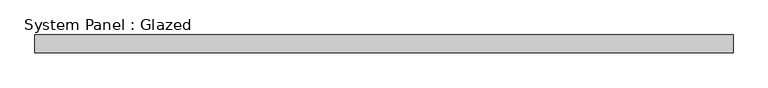
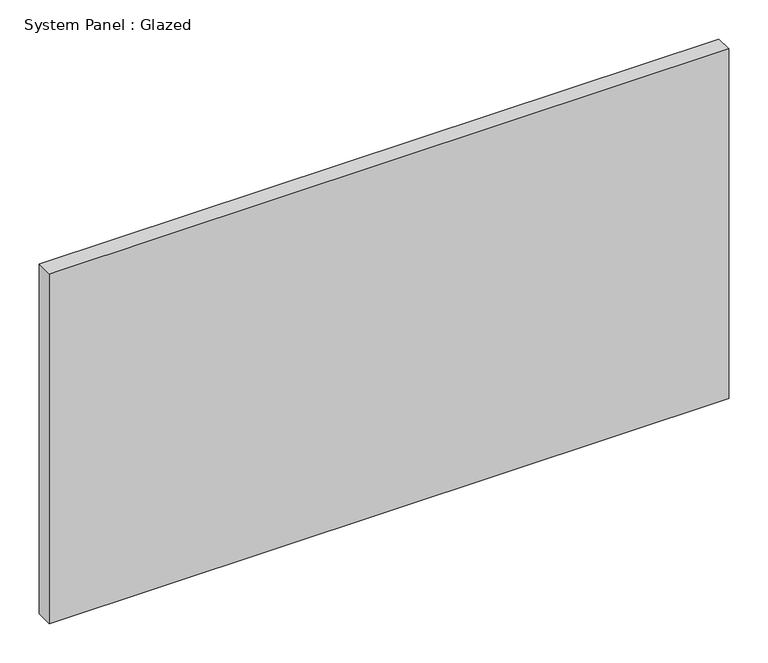
"""IFC4 building model written with IfcOpenShell, lengths in millimetres: plate geometry, System Panel : Glazed."""

from ifc_helpers import new_model, si_unit, origin, origin_with_axes, place, context, project, spatial, polyline, outline, extrude, source, transform, mapped, element, save


def system_panel_glazed_c1629c18(model_context):
    return source(origin(), model_context, "Body", "SweptSolid", [
        extrude(outline(polyline([(501.65, 19.05), (-501.65, 19.05), (-501.65, 44.45), (501.65, 44.45), (501.65, 19.05)])), origin_with_axes(), (0.0, 0.0, 1.0), 546.1),
    ])


if __name__ == "__main__":
    model = new_model("IFC4")
    model_context = context("Model", 3, world=origin())
    ifc_project = project(units=[si_unit("LENGTHUNIT", "METRE", prefix="MILLI")], contexts=[model_context])
    site = spatial("IfcSite", under=ifc_project)
    building = spatial("IfcBuilding", under=site)
    placement = place(None, origin())
    system_panel_glazed_shape = system_panel_glazed_c1629c18(model_context)
    element("IfcPlate", 1, ObjectType="System Panel : Glazed", at=placement, inside=building, context=model_context, shape_type="MappedRepresentation", body=[
        mapped(system_panel_glazed_shape, transform((0.0, 0.0, 0.0), x_axis=(1.0, 0.0, 0.0), y_axis=(0.0, 1.0, 0.0), z_axis=(0.0, 0.0, 1.0))),
    ])
    save(model, "model.ifc")

# Revit data of these elements
# Type "System Panel : Glazed"
#   Construction Type Id = "GSP4R"
#   Analytic Construction = "1/8 in Pilkington single glazing"
#   Visual Light Transmittance = 0.9
#   Solar Heat Gain Coefficient = 0.86
#   Heat Transfer Coefficient (U) = 1.18115 BTU/(h·ft²·°F)
# Element 1 (IfcPlate, "System Panel : Glazed")
#   Materials on its faces: "Glass"
# Materials
#   "Glass": class "Glass", colour RGB 0 128 192, transparency 0.75, Description = "Soda Lime Glass", Cost = 0
